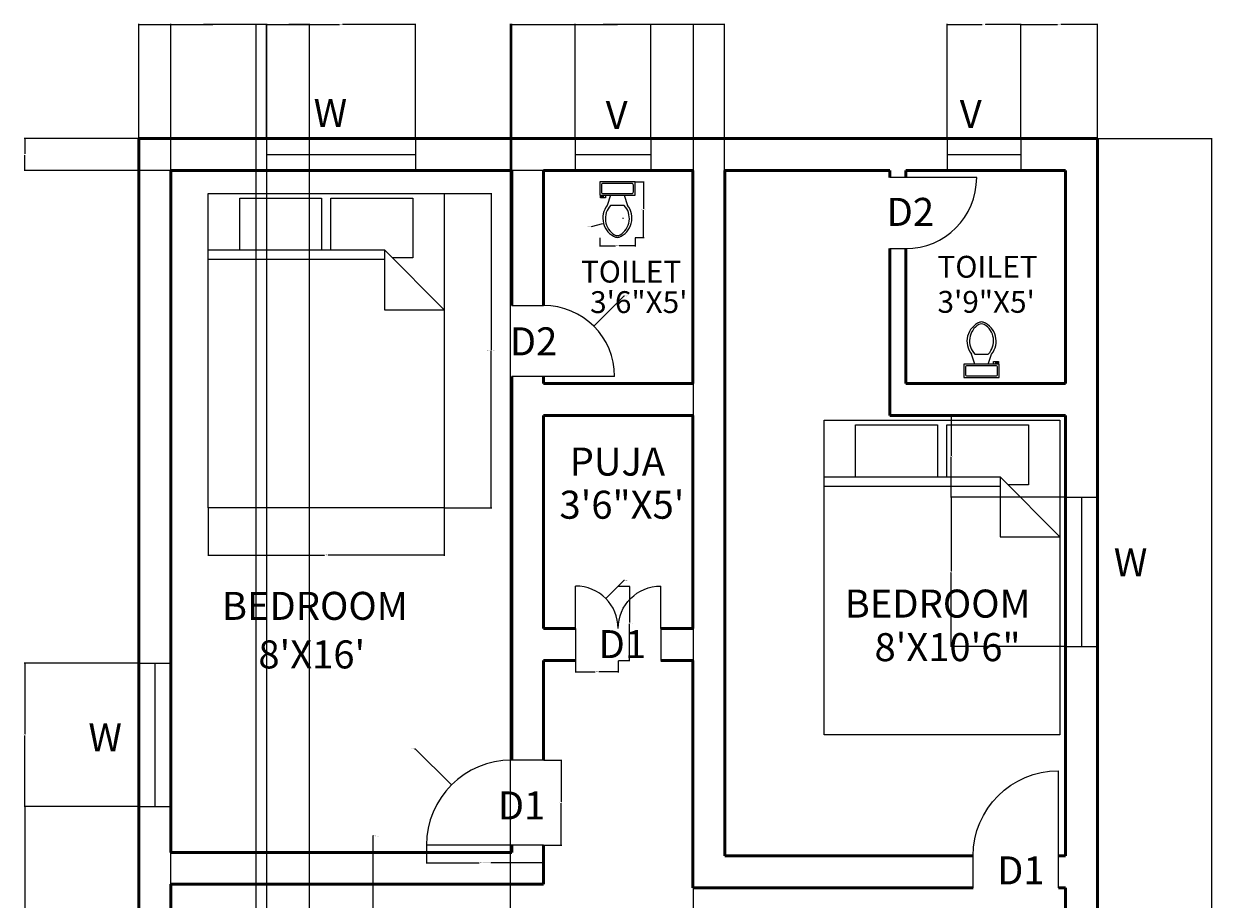
# Model space of a CAD drawing. Units: feet. Extents: x 1657 to 2001, y 1678 to 2367.
# Tile 4 of 4: x 1666 to 2001, y 2120 to 2367. Entities that reach past the tile are written whole.
import ezdxf

# ---------------------------------------------------------------- set-up
doc = ezdxf.new("R2010")
doc.units = ezdxf.units.FT
for name, color, linetype, lineweight in [('A-ANNO-DIMS', 2, 'Continuous', 18), ('A-ANNO-TEXT', 7, 'Continuous', 18), ('A-AREA-IDEN', 7, 'Continuous', 25), ('A-DOOR', 3, 'Continuous', 25), ('A-FLOR-FIXT', 8, 'Continuous', 18), ('A-FURN', 8, 'Continuous', 18), ('A-GLAZ', 4, 'Continuous', 18), ('A-WALL', 7, 'Continuous', 50)]:
    doc.layers.add(name, color=color, linetype=linetype, lineweight=lineweight)
doc.styles.get("Standard").update_dxf_attribs({"font": 'arial.ttf'})
doc.dimstyles.get("Standard").update_dxf_attribs({"dimtxt": 0.18, "dimasz": 0.18, "dimexe": 0.18, "dimexo": 0.0625, "dimgap": 0.09, "dimtad": 0, "dimtih": 1, "dimtoh": 1, "dimdec": 4, "dimzin": 0, "dimdsep": 46, "dimtxsty": 'Standard', "dimcen": 0.09, "dimadec": 0, "dimazin": 0, "dimtfac": 1, "dimtdec": 4, "dimtofl": 0, "dimtmove": 0, "dimatfit": 3, "dimfxl": 1, "dimtolj": 1, "dimtzin": 0, "dimarcsym": 0})

# ---------------------------------------------------------------- blocks, each defined once
blk = doc.blocks.new('Bed - Queen')
for p, q in [((0, -80.00003), (0, 0)), ((0, 0), (59.99999, 0)), ((59.99999, 0), (59.99999, -80.00003)), ((7.99999, -1.2), (28.79998, -1.2)), ((7.99999, -14.4), (7.99999, -1.2)), ((28.79998, -1.2), (28.79998, -14.4)), ((31.19999, -1.2), (51.99999, -1.2)), ((31.19999, -14.4), (31.19999, -1.2)), ((51.99999, -1.2), (51.99999, -16.4)), ((0, -14.4), (44.8, -14.4)), ((59.99999, -29.6), (44.8, -14.4)), ((44.8, -14.4), (44.8, -29.6)), ((44.8, -16.8), (0, -16.8)), ((51.99999, -16.4), (46.79936, -16.4)), ((44.8, -29.6), (59.99999, -29.6)), ((59.99999, -80.00003), (0, -80.00003))]:
    blk.add_line(p, q)
blk = doc.blocks.new('Toilet - top')
for p, q in [((9.5, -6), (9.5, -2)), ((-10, -8.5), (-8, -8.5)), ((-10, -9.5), (-10, -8.5)), ((-7, -9.5), (-10, -9.5)), ((-8, -8.5), (-8, -8)), ((-7, -8), (-7, -9.5)), ((-4, -8), (-6, -14)), ((4, -14), (-4, -14)), ((4, -8), (6, -14))]:
    blk.add_line(p, q)
blk.add_lwpolyline([(10.5, -8), (10.5, 0), (-10.5, 0), (-10.5, -8)], close=True)
for points in [[(-9.5, -2), (-9.5, -6)], [(8.5, -1), (-8.5, -1)], [(-8.5, -7), (8.5, -7)]]:
    blk.add_lwpolyline(points)
for centre, radius, start, end in [((-8.62, -1.88), 0.884, 81.8699, 188.1301), ((-8.62, -6.12), 0.884, 171.8699, 278.1301), ((8.62, -1.88), 0.884, 351.8699, 98.1301), ((8.62, -6.12), 0.884, 261.8699, 8.1301), ((3.52, -21.58), 12.17, 141.46911, 247.97143), ((4.2, -21.82), 11.33, 136.36773, 238.94682), ((-3.52, -21.58), 12.17, 292.02843, 38.53071), ((-4.2, -21.82), 11.33, 301.05301, 43.63209), ((0, -27.88), 4, 245.73182, 294.26817), ((0, -29), 4, 254.86053, 285.13947)]:
    blk.add_arc(centre, radius, start, end)
blk = doc.blocks.new('DOOR-BEDROOM-SINGLE')
for p, q in [((33, 24), (24, 24)), ((33, 0), (0, 0))]:
    blk.add_line(p, q)
blk.add_arc((24, 0), 24, 90, 180)
blk = doc.blocks.new('DOOR-PUJA-LEAF')
for q in [(0, 21), (0, 0)]:
    blk.add_line((0, 9), q)
blk.add_arc((0, 9), 12, 0, 90)
blk = doc.blocks.new('*D12')
at = {"layer": 'A-ANNO-DIMS', "color": 0, "lineweight": -2, "transparency": 16777216}
for p, q in [((1784.32, 2318.87), (1797.72, 2318.87)), ((1797.54, 2318.69), (1797.54, 2274.76)), ((1797.54, 2230.46), (1797.54, 2274.39)), ((1784.32, 2230.28), (1797.72, 2230.28))]:
    blk.add_line(p, q, dxfattribs=at)
at = {"layer": 'A-ANNO-DIMS', "color": 0, "transparency": 16777216}
for points in [[(1797.51, 2318.69), (1797.57, 2318.69), (1797.54, 2318.87)], [(1797.51, 2230.46), (1797.57, 2230.46), (1797.54, 2230.28)]]:
    blk.add_solid(points, dxfattribs=at)
at = {"layer": 'Defpoints', "color": 0, "transparency": 16777216}
for p in [(1784.26, 2318.87), (1797.54, 2318.87), (1784.26, 2230.28)]:
    blk.add_point(p, dxfattribs=at)
at = {"layer": 'A-ANNO-DIMS', "color": 0, "transparency": 16777216, "insert": (1797.54, 2274.57), "char_height": 0.18, "attachment_point": 5}
blk.add_mtext('\\A1;QUEEN BED 89 TYP.', dxfattribs=at)
blk = doc.blocks.new('*D13')
at = {"layer": 'A-ANNO-DIMS', "color": 0, "lineweight": -2, "transparency": 16777216}
for p, q in [((1717.81, 2230.22), (1717.81, 2216.81)), ((1784.26, 2230.22), (1784.26, 2216.81)), ((1717.99, 2216.99), (1750.51, 2216.99)), ((1784.08, 2216.99), (1751.56, 2216.99))]:
    blk.add_line(p, q, dxfattribs=at)
at = {"layer": 'A-ANNO-DIMS', "color": 0, "transparency": 16777216}
for points in [[(1717.99, 2217.02), (1717.99, 2216.96), (1717.81, 2216.99)], [(1784.08, 2217.02), (1784.08, 2216.96), (1784.26, 2216.99)]]:
    blk.add_solid(points, dxfattribs=at)
at = {"layer": 'Defpoints', "color": 0, "transparency": 16777216}
for p in [(1717.81, 2230.28), (1784.26, 2230.28), (1784.26, 2216.99)]:
    blk.add_point(p, dxfattribs=at)
at = {"layer": 'A-ANNO-DIMS', "color": 0, "transparency": 16777216, "insert": (1751.03, 2216.99), "char_height": 0.18, "attachment_point": 5}
blk.add_mtext('\\A1;66 TYP.', dxfattribs=at)
blk = doc.blocks.new('*D14')
at = {"layer": 'A-ANNO-DIMS', "color": 0, "lineweight": -2, "transparency": 16777216}
for p, q in [((1838.1, 2322.14), (1840.57, 2322.14)), ((1840.39, 2321.96), (1840.39, 2314.48)), ((1840.39, 2306.63), (1840.39, 2314.11)), ((1838.1, 2306.45), (1840.57, 2306.45))]:
    blk.add_line(p, q, dxfattribs=at)
at = {"layer": 'A-ANNO-DIMS', "color": 0, "transparency": 16777216}
for points in [[(1840.36, 2321.96), (1840.42, 2321.96), (1840.39, 2322.14)], [(1840.36, 2306.63), (1840.42, 2306.63), (1840.39, 2306.45)]]:
    blk.add_solid(points, dxfattribs=at)
at = {"layer": 'Defpoints', "color": 0, "transparency": 16777216}
for p in [(1838.04, 2322.14), (1840.39, 2322.14), (1838.04, 2306.45)]:
    blk.add_point(p, dxfattribs=at)
at = {"layer": 'A-ANNO-DIMS', "color": 0, "transparency": 16777216, "insert": (1840.39, 2314.3), "char_height": 0.18, "attachment_point": 5}
blk.add_mtext('\\A1;WC 16 TYP.', dxfattribs=at)
blk = doc.blocks.new('*D15')
at = {"layer": 'A-ANNO-DIMS', "color": 0, "lineweight": -2, "transparency": 16777216}
for p, q in [((1828.07, 2306.39), (1828.07, 2303.92)), ((1828.25, 2304.1), (1832.54, 2304.1)), ((1837.86, 2304.1), (1833.58, 2304.1)), ((1838.04, 2306.39), (1838.04, 2303.92))]:
    blk.add_line(p, q, dxfattribs=at)
at = {"layer": 'A-ANNO-DIMS', "color": 0, "transparency": 16777216}
for points in [[(1828.25, 2304.13), (1828.25, 2304.07), (1828.07, 2304.1)], [(1837.86, 2304.13), (1837.86, 2304.07), (1838.04, 2304.1)]]:
    blk.add_solid(points, dxfattribs=at)
at = {"layer": 'Defpoints', "color": 0, "transparency": 16777216}
for p in [(1828.07, 2306.45), (1838.04, 2306.45), (1838.04, 2304.1)]:
    blk.add_point(p, dxfattribs=at)
at = {"layer": 'A-ANNO-DIMS', "color": 0, "transparency": 16777216, "insert": (1833.06, 2304.1), "char_height": 0.18, "attachment_point": 5}
blk.add_mtext('\\A1;10 TYP.', dxfattribs=at)
blk = doc.blocks.new('*D28')
at = {"layer": 'A-ANNO-DIMS', "color": 0, "lineweight": -2, "transparency": 16777216}
for p, q in [((1779.28, 2135.24), (1779.28, 2130.17)), ((1812.28, 2135.24), (1812.28, 2130.17)), ((1779.46, 2130.35), (1794.16, 2130.35)), ((1812.1, 2130.35), (1797.41, 2130.35))]:
    blk.add_line(p, q, dxfattribs=at)
at = {"layer": 'A-ANNO-DIMS', "color": 0, "transparency": 16777216}
for points in [[(1779.46, 2130.38), (1779.46, 2130.32), (1779.28, 2130.35)], [(1812.1, 2130.38), (1812.1, 2130.32), (1812.28, 2130.35)]]:
    blk.add_solid(points, dxfattribs=at)
at = {"layer": 'Defpoints', "color": 0, "transparency": 16777216}
for p in [(1779.28, 2135.3), (1812.28, 2135.3), (1812.28, 2130.35)]:
    blk.add_point(p, dxfattribs=at)
at = {"layer": 'A-ANNO-DIMS', "color": 0, "transparency": 16777216, "insert": (1795.78, 2130.35), "char_height": 0.18, "attachment_point": 5}
blk.add_mtext('\\A1;BEDROOM DOOR 33 TYP.', dxfattribs=at)
blk = doc.blocks.new('*D29')
at = {"layer": 'A-ANNO-DIMS', "color": 0, "lineweight": -2, "transparency": 16777216}
for p, q in [((1812.35, 2159.3), (1817.41, 2159.3)), ((1817.23, 2159.12), (1817.23, 2147.48)), ((1817.23, 2135.48), (1817.23, 2147.12)), ((1812.35, 2135.3), (1817.41, 2135.3))]:
    blk.add_line(p, q, dxfattribs=at)
at = {"layer": 'A-ANNO-DIMS', "color": 0, "transparency": 16777216}
for points in [[(1817.2, 2159.12), (1817.26, 2159.12), (1817.23, 2159.3)], [(1817.2, 2135.48), (1817.26, 2135.48), (1817.23, 2135.3)]]:
    blk.add_solid(points, dxfattribs=at)
at = {"layer": 'Defpoints', "color": 0, "transparency": 16777216}
for p in [(1812.28, 2159.3), (1817.23, 2159.3), (1812.28, 2135.3)]:
    blk.add_point(p, dxfattribs=at)
at = {"layer": 'A-ANNO-DIMS', "color": 0, "transparency": 16777216, "insert": (1817.23, 2147.3), "char_height": 0.18, "attachment_point": 5}
blk.add_mtext('\\A1;24 TYP.', dxfattribs=at)
blk = doc.blocks.new('*D32')
at = {"layer": 'A-ANNO-DIMS', "color": 0, "lineweight": -2, "transparency": 16777216}
for p, q in [((1833.35, 2208.3), (1836.61, 2208.3)), ((1836.43, 2208.12), (1836.43, 2197.98)), ((1836.43, 2187.48), (1836.43, 2197.62)), ((1833.35, 2187.3), (1836.61, 2187.3))]:
    blk.add_line(p, q, dxfattribs=at)
at = {"layer": 'A-ANNO-DIMS', "color": 0, "transparency": 16777216}
for points in [[(1836.4, 2208.12), (1836.46, 2208.12), (1836.43, 2208.3)], [(1836.4, 2187.48), (1836.46, 2187.48), (1836.43, 2187.3)]]:
    blk.add_solid(points, dxfattribs=at)
at = {"layer": 'Defpoints', "color": 0, "transparency": 16777216}
for p in [(1833.28, 2208.3), (1836.43, 2208.3), (1833.28, 2187.3)]:
    blk.add_point(p, dxfattribs=at)
at = {"layer": 'A-ANNO-DIMS', "color": 0, "transparency": 16777216, "insert": (1836.43, 2197.8), "char_height": 0.18, "attachment_point": 5}
blk.add_mtext('\\A1;PUJA LEAF 21 TYP.', dxfattribs=at)
blk = doc.blocks.new('*D33')
at = {"layer": 'A-ANNO-DIMS', "color": 0, "lineweight": -2, "transparency": 16777216}
for p, q in [((1821.28, 2187.24), (1821.28, 2183.97)), ((1833.28, 2187.24), (1833.28, 2183.97)), ((1821.46, 2184.15), (1826.77, 2184.15)), ((1833.1, 2184.15), (1827.8, 2184.15))]:
    blk.add_line(p, q, dxfattribs=at)
at = {"layer": 'A-ANNO-DIMS', "color": 0, "transparency": 16777216}
for points in [[(1821.46, 2184.18), (1821.46, 2184.12), (1821.28, 2184.15)], [(1833.1, 2184.18), (1833.1, 2184.12), (1833.28, 2184.15)]]:
    blk.add_solid(points, dxfattribs=at)
at = {"layer": 'Defpoints', "color": 0, "transparency": 16777216}
for p in [(1821.28, 2187.3), (1833.28, 2187.3), (1833.28, 2184.15)]:
    blk.add_point(p, dxfattribs=at)
at = {"layer": 'A-ANNO-DIMS', "color": 0, "transparency": 16777216, "insert": (1827.28, 2184.15), "char_height": 0.18, "attachment_point": 5}
blk.add_mtext('\\A1;12 TYP.', dxfattribs=at)
blk = doc.blocks.new('*D35')
at = {"layer": 'A-ANNO-DIMS', "color": 0, "lineweight": -2, "transparency": 16777216}
for p, q in [((1968.35, 2334.3), (2000.61, 2334.3)), ((2000.43, 2334.12), (2000.43, 2022.48)), ((2000.43, 1710.48), (2000.43, 2022.12)), ((1968.35, 1710.3), (2000.61, 1710.3))]:
    blk.add_line(p, q, dxfattribs=at)
at = {"layer": 'A-ANNO-DIMS', "color": 0, "transparency": 16777216}
for points in [[(2000.4, 2334.12), (2000.46, 2334.12), (2000.43, 2334.3)], [(2000.4, 1710.48), (2000.46, 1710.48), (2000.43, 1710.3)]]:
    blk.add_solid(points, dxfattribs=at)
at = {"layer": 'Defpoints', "color": 0, "transparency": 16777216}
for p in [(1968.28, 2334.3), (2000.43, 2334.3), (1968.28, 1710.3)]:
    blk.add_point(p, dxfattribs=at)
at = {"layer": 'A-ANNO-DIMS', "color": 0, "transparency": 16777216, "insert": (2000.43, 2022.3), "char_height": 0.18, "attachment_point": 5}
blk.add_mtext('\\A1;624', dxfattribs=at)
blk = doc.blocks.new('*D37')
at = {"layer": 'A-ANNO-DIMS', "color": 0, "lineweight": -2, "transparency": 16777216}
for p, q in [((1734.28, 1770.36), (1734.28, 2366.63)), ((1734.46, 2366.45), (1740.08, 2366.45)), ((1746.1, 2366.45), (1740.49, 2366.45)), ((1746.28, 1770.36), (1746.28, 2366.63))]:
    blk.add_line(p, q, dxfattribs=at)
at = {"layer": 'A-ANNO-DIMS', "color": 0, "transparency": 16777216}
for points in [[(1734.46, 2366.48), (1734.46, 2366.42), (1734.28, 2366.45)], [(1746.1, 2366.48), (1746.1, 2366.42), (1746.28, 2366.45)]]:
    blk.add_solid(points, dxfattribs=at)
at = {"layer": 'Defpoints', "color": 0, "transparency": 16777216}
for p in [(1746.28, 2366.45), (1734.28, 1770.3), (1746.28, 1770.3)]:
    blk.add_point(p, dxfattribs=at)
at = {"layer": 'A-ANNO-DIMS', "color": 0, "transparency": 16777216, "insert": (1740.28, 2366.45), "char_height": 0.18, "attachment_point": 5}
blk.add_mtext('\\A1;12', dxfattribs=at)
blk = doc.blocks.new('*D38')
at = {"layer": 'A-ANNO-DIMS', "color": 0, "lineweight": -2, "transparency": 16777216}
for p, q in [((1698.28, 1770.36), (1698.28, 2366.63)), ((1698.46, 2366.45), (1716.07, 2366.45)), ((1734.1, 2366.45), (1716.5, 2366.45)), ((1734.28, 1770.36), (1734.28, 2366.63))]:
    blk.add_line(p, q, dxfattribs=at)
at = {"layer": 'A-ANNO-DIMS', "color": 0, "transparency": 16777216}
for points in [[(1698.46, 2366.48), (1698.46, 2366.42), (1698.28, 2366.45)], [(1734.1, 2366.48), (1734.1, 2366.42), (1734.28, 2366.45)]]:
    blk.add_solid(points, dxfattribs=at)
at = {"layer": 'Defpoints', "color": 0, "transparency": 16777216}
for p in [(1734.28, 2366.45), (1698.28, 1770.3), (1734.28, 1770.3)]:
    blk.add_point(p, dxfattribs=at)
at = {"layer": 'A-ANNO-DIMS', "color": 0, "transparency": 16777216, "insert": (1716.28, 2366.45), "char_height": 0.18, "attachment_point": 5}
blk.add_mtext('\\A1;36', dxfattribs=at)
blk = doc.blocks.new('*D39')
at = {"layer": 'A-ANNO-DIMS', "color": 0, "lineweight": -2, "transparency": 16777216}
for p, q in [((1698.28, 2334.36), (1698.28, 2366.63)), ((1698.46, 2366.45), (1715.79, 2366.45)), ((1734.04, 2366.45), (1716.72, 2366.45)), ((1734.22, 2334.36), (1734.22, 2366.63))]:
    blk.add_line(p, q, dxfattribs=at)
at = {"layer": 'A-ANNO-DIMS', "color": 0, "transparency": 16777216}
for points in [[(1698.46, 2366.48), (1698.46, 2366.42), (1698.28, 2366.45)], [(1734.04, 2366.48), (1734.04, 2366.42), (1734.22, 2366.45)]]:
    blk.add_solid(points, dxfattribs=at)
at = {"layer": 'Defpoints', "color": 0, "transparency": 16777216}
for p in [(1734.22, 2366.45), (1698.28, 2334.3), (1734.22, 2334.3)]:
    blk.add_point(p, dxfattribs=at)
at = {"layer": 'A-ANNO-DIMS', "color": 0, "transparency": 16777216, "insert": (1716.25, 2366.45), "char_height": 0.18, "attachment_point": 5}
blk.add_mtext('\\A1;35.935', dxfattribs=at)
blk = doc.blocks.new('*D40')
at = {"layer": 'A-ANNO-DIMS', "color": 0, "lineweight": -2, "transparency": 16777216}
for p, q in [((1734.22, 2334.36), (1734.22, 2366.63)), ((1734.4, 2366.45), (1754.79, 2366.45)), ((1775.98, 2366.45), (1755.59, 2366.45)), ((1776.16, 2334.36), (1776.16, 2366.63))]:
    blk.add_line(p, q, dxfattribs=at)
at = {"layer": 'A-ANNO-DIMS', "color": 0, "transparency": 16777216}
for points in [[(1734.4, 2366.48), (1734.4, 2366.42), (1734.22, 2366.45)], [(1775.98, 2366.48), (1775.98, 2366.42), (1776.16, 2366.45)]]:
    blk.add_solid(points, dxfattribs=at)
at = {"layer": 'Defpoints', "color": 0, "transparency": 16777216}
for p in [(1776.16, 2366.45), (1734.22, 2334.3), (1776.16, 2334.3)]:
    blk.add_point(p, dxfattribs=at)
at = {"layer": 'A-ANNO-DIMS', "color": 0, "transparency": 16777216, "insert": (1755.19, 2366.45), "char_height": 0.18, "attachment_point": 5}
blk.add_mtext('\\A1;41.94', dxfattribs=at)
blk = doc.blocks.new('*D41')
at = {"layer": 'A-ANNO-DIMS', "color": 0, "lineweight": -2, "transparency": 16777216}
for p, q in [((1925.97, 2334.36), (1925.97, 2366.63)), ((1926.15, 2366.45), (1935.87, 2366.45)), ((1946.52, 2366.45), (1936.8, 2366.45)), ((1946.7, 2334.36), (1946.7, 2366.63))]:
    blk.add_line(p, q, dxfattribs=at)
at = {"layer": 'A-ANNO-DIMS', "color": 0, "transparency": 16777216}
for points in [[(1926.15, 2366.48), (1926.15, 2366.42), (1925.97, 2366.45)], [(1946.52, 2366.48), (1946.52, 2366.42), (1946.7, 2366.45)]]:
    blk.add_solid(points, dxfattribs=at)
at = {"layer": 'Defpoints', "color": 0, "transparency": 16777216}
for p in [(1946.7, 2366.45), (1925.97, 2334.3), (1946.7, 2334.3)]:
    blk.add_point(p, dxfattribs=at)
at = {"layer": 'A-ANNO-DIMS', "color": 0, "transparency": 16777216, "insert": (1936.33, 2366.45), "char_height": 0.18, "attachment_point": 5}
blk.add_mtext('\\A1;20.726', dxfattribs=at)
blk = doc.blocks.new('*D42')
at = {"layer": 'A-ANNO-DIMS', "color": 0, "lineweight": -2, "transparency": 16777216}
for p, q in [((1946.7, 2334.36), (1946.7, 2366.63)), ((1946.88, 2366.45), (1957.03, 2366.45)), ((1968.1, 2366.45), (1957.96, 2366.45)), ((1968.28, 2334.36), (1968.28, 2366.63))]:
    blk.add_line(p, q, dxfattribs=at)
at = {"layer": 'A-ANNO-DIMS', "color": 0, "transparency": 16777216}
for points in [[(1946.88, 2366.48), (1946.88, 2366.42), (1946.7, 2366.45)], [(1968.1, 2366.48), (1968.1, 2366.42), (1968.28, 2366.45)]]:
    blk.add_solid(points, dxfattribs=at)
at = {"layer": 'Defpoints', "color": 0, "transparency": 16777216}
for p in [(1968.28, 2366.45), (1946.7, 2334.3), (1968.28, 2334.3)]:
    blk.add_point(p, dxfattribs=at)
at = {"layer": 'A-ANNO-DIMS', "color": 0, "transparency": 16777216, "insert": (1957.49, 2366.45), "char_height": 0.18, "attachment_point": 5}
blk.add_mtext('\\A1;21.588', dxfattribs=at)
blk = doc.blocks.new('*D46')
at = {"layer": 'A-ANNO-DIMS', "color": 0, "lineweight": -2, "transparency": 16777216}
for p, q in [((1698.22, 2146.17), (1665.95, 2146.17)), ((1666.13, 2145.99), (1666.13, 2111.13)), ((1666.13, 2075.91), (1666.13, 2110.77)), ((1698.22, 2075.73), (1665.95, 2075.73))]:
    blk.add_line(p, q, dxfattribs=at)
at = {"layer": 'A-ANNO-DIMS', "color": 0, "transparency": 16777216}
for points in [[(1666.1, 2145.99), (1666.16, 2145.99), (1666.13, 2146.17)], [(1666.1, 2075.91), (1666.16, 2075.91), (1666.13, 2075.73)]]:
    blk.add_solid(points, dxfattribs=at)
at = {"layer": 'Defpoints', "color": 0, "transparency": 16777216}
for p in [(1666.13, 2146.17), (1698.28, 2146.17), (1698.28, 2075.73)]:
    blk.add_point(p, dxfattribs=at)
at = {"layer": 'A-ANNO-DIMS', "color": 0, "transparency": 16777216, "insert": (1666.13, 2110.95), "char_height": 0.18, "attachment_point": 5}
blk.add_mtext('\\A1;70.44', dxfattribs=at)
blk = doc.blocks.new('*D47')
at = {"layer": 'A-ANNO-DIMS', "color": 0, "lineweight": -2, "transparency": 16777216}
for p, q in [((1698.22, 2186.61), (1665.95, 2186.61)), ((1666.13, 2186.43), (1666.13, 2166.57)), ((1666.13, 2146.35), (1666.13, 2166.21)), ((1698.22, 2146.17), (1665.95, 2146.17))]:
    blk.add_line(p, q, dxfattribs=at)
at = {"layer": 'A-ANNO-DIMS', "color": 0, "transparency": 16777216}
for points in [[(1666.1, 2186.43), (1666.16, 2186.43), (1666.13, 2186.61)], [(1666.1, 2146.35), (1666.16, 2146.35), (1666.13, 2146.17)]]:
    blk.add_solid(points, dxfattribs=at)
at = {"layer": 'Defpoints', "color": 0, "transparency": 16777216}
for p in [(1666.13, 2186.61), (1698.28, 2186.61), (1698.28, 2146.17)]:
    blk.add_point(p, dxfattribs=at)
at = {"layer": 'A-ANNO-DIMS', "color": 0, "transparency": 16777216, "insert": (1666.13, 2166.39), "char_height": 0.18, "attachment_point": 5}
blk.add_mtext('\\A1;40.45', dxfattribs=at)
blk = doc.blocks.new('*D48')
at = {"layer": 'A-ANNO-DIMS', "color": 0, "lineweight": -2, "transparency": 16777216}
for p, q in [((1959.22, 2233.29), (1926.95, 2233.29)), ((1927.13, 2233.11), (1927.13, 2212.44)), ((1927.13, 2191.4), (1927.13, 2212.07)), ((1959.22, 2191.22), (1926.95, 2191.22))]:
    blk.add_line(p, q, dxfattribs=at)
at = {"layer": 'A-ANNO-DIMS', "color": 0, "transparency": 16777216}
for points in [[(1927.1, 2233.11), (1927.16, 2233.11), (1927.13, 2233.29)], [(1927.1, 2191.4), (1927.16, 2191.4), (1927.13, 2191.22)]]:
    blk.add_solid(points, dxfattribs=at)
at = {"layer": 'Defpoints', "color": 0, "transparency": 16777216}
for p in [(1927.13, 2233.29), (1959.28, 2233.29), (1959.28, 2191.22)]:
    blk.add_point(p, dxfattribs=at)
at = {"layer": 'A-ANNO-DIMS', "color": 0, "transparency": 16777216, "insert": (1927.13, 2212.26), "char_height": 0.18, "attachment_point": 5}
blk.add_mtext('\\A1;42.06', dxfattribs=at)
blk = doc.blocks.new('*D49')
at = {"layer": 'A-ANNO-DIMS', "color": 0, "lineweight": -2, "transparency": 16777216}
for p, q in [((1959.22, 2256.3), (1926.95, 2256.3)), ((1927.13, 2256.12), (1927.13, 2244.97)), ((1927.13, 2233.47), (1927.13, 2244.61)), ((1959.22, 2233.29), (1926.95, 2233.29))]:
    blk.add_line(p, q, dxfattribs=at)
at = {"layer": 'A-ANNO-DIMS', "color": 0, "transparency": 16777216}
for points in [[(1927.1, 2256.12), (1927.16, 2256.12), (1927.13, 2256.3)], [(1927.1, 2233.47), (1927.16, 2233.47), (1927.13, 2233.29)]]:
    blk.add_solid(points, dxfattribs=at)
at = {"layer": 'Defpoints', "color": 0, "transparency": 16777216}
for p in [(1927.13, 2256.3), (1959.28, 2256.3), (1959.28, 2233.29)]:
    blk.add_point(p, dxfattribs=at)
at = {"layer": 'A-ANNO-DIMS', "color": 0, "transparency": 16777216, "insert": (1927.13, 2244.79), "char_height": 0.18, "attachment_point": 5}
blk.add_mtext('\\A1;23.01', dxfattribs=at)
blk = doc.blocks.new('*D50')
at = {"layer": 'A-ANNO-DIMS', "color": 0, "lineweight": -2, "transparency": 16777216}
for p, q in [((1803.28, 2325.36), (1803.28, 2366.63)), ((1803.46, 2366.45), (1833.07, 2366.45)), ((1863.1, 2366.45), (1833.5, 2366.45)), ((1863.28, 2325.36), (1863.28, 2366.63))]:
    blk.add_line(p, q, dxfattribs=at)
at = {"layer": 'A-ANNO-DIMS', "color": 0, "transparency": 16777216}
for points in [[(1803.46, 2366.48), (1803.46, 2366.42), (1803.28, 2366.45)], [(1863.1, 2366.48), (1863.1, 2366.42), (1863.28, 2366.45)]]:
    blk.add_solid(points, dxfattribs=at)
at = {"layer": 'Defpoints', "color": 0, "transparency": 16777216}
for p in [(1863.28, 2366.45), (1803.28, 2325.3), (1863.28, 2325.3)]:
    blk.add_point(p, dxfattribs=at)
at = {"layer": 'A-ANNO-DIMS', "color": 0, "transparency": 16777216, "insert": (1833.28, 2366.45), "char_height": 0.18, "attachment_point": 5}
blk.add_mtext('\\A1;60', dxfattribs=at)
blk = doc.blocks.new('*D51')
at = {"layer": 'A-ANNO-DIMS', "color": 0, "lineweight": -2, "transparency": 16777216}
for p, q in [((1821.17, 2334.36), (1821.17, 2366.63)), ((1821.35, 2366.45), (1831.45, 2366.45)), ((1842.34, 2366.45), (1832.24, 2366.45)), ((1842.52, 2334.36), (1842.52, 2366.63))]:
    blk.add_line(p, q, dxfattribs=at)
at = {"layer": 'A-ANNO-DIMS', "color": 0, "transparency": 16777216}
for points in [[(1821.35, 2366.48), (1821.35, 2366.42), (1821.17, 2366.45)], [(1842.34, 2366.48), (1842.34, 2366.42), (1842.52, 2366.45)]]:
    blk.add_solid(points, dxfattribs=at)
at = {"layer": 'Defpoints', "color": 0, "transparency": 16777216}
for p in [(1842.52, 2366.45), (1821.17, 2334.3), (1842.52, 2334.3)]:
    blk.add_point(p, dxfattribs=at)
at = {"layer": 'A-ANNO-DIMS', "color": 0, "transparency": 16777216, "insert": (1831.85, 2366.45), "char_height": 0.18, "attachment_point": 5}
blk.add_mtext('\\A1;21.35', dxfattribs=at)
blk = doc.blocks.new('*D52')
at = {"layer": 'A-ANNO-DIMS', "color": 0, "lineweight": -2, "transparency": 16777216}
for p, q in [((1821.11, 2334.3), (1665.95, 2334.3)), ((1666.13, 2334.12), (1666.13, 2329.98)), ((1666.13, 2325.48), (1666.13, 2329.62)), ((1821.11, 2325.3), (1665.95, 2325.3))]:
    blk.add_line(p, q, dxfattribs=at)
at = {"layer": 'A-ANNO-DIMS', "color": 0, "transparency": 16777216}
for points in [[(1666.1, 2334.12), (1666.16, 2334.12), (1666.13, 2334.3)], [(1666.1, 2325.48), (1666.16, 2325.48), (1666.13, 2325.3)]]:
    blk.add_solid(points, dxfattribs=at)
at = {"layer": 'Defpoints', "color": 0, "transparency": 16777216}
for p in [(1821.17, 2334.3), (1666.13, 2325.3), (1821.17, 2325.3)]:
    blk.add_point(p, dxfattribs=at)
at = {"layer": 'A-ANNO-DIMS', "color": 0, "transparency": 16777216, "insert": (1666.13, 2329.8), "char_height": 0.18, "attachment_point": 5}
blk.add_mtext('\\A1;9', dxfattribs=at)
blk = doc.blocks.new('*D55')
at = {"layer": 'A-ANNO-DIMS', "color": 0, "lineweight": -2, "transparency": 16777216}
for p, q in [((1707.28, 1851.36), (1707.28, 2366.63)), ((1707.46, 2366.45), (1719.06, 2366.45)), ((1731.1, 2366.45), (1719.5, 2366.45)), ((1731.28, 1851.36), (1731.28, 2366.63))]:
    blk.add_line(p, q, dxfattribs=at)
at = {"layer": 'A-ANNO-DIMS', "color": 0, "transparency": 16777216}
for points in [[(1707.46, 2366.48), (1707.46, 2366.42), (1707.28, 2366.45)], [(1731.1, 2366.48), (1731.1, 2366.42), (1731.28, 2366.45)]]:
    blk.add_solid(points, dxfattribs=at)
at = {"layer": 'Defpoints', "color": 0, "transparency": 16777216}
for p in [(1731.28, 2366.45), (1707.28, 1851.3), (1731.28, 1851.3)]:
    blk.add_point(p, dxfattribs=at)
at = {"layer": 'A-ANNO-DIMS', "color": 0, "transparency": 16777216, "insert": (1719.28, 2366.45), "char_height": 0.18, "attachment_point": 5}
blk.add_mtext('\\A1;24', dxfattribs=at)
blk = doc.blocks.new('*D56')
at = {"layer": 'A-ANNO-DIMS', "color": 0, "lineweight": -2, "transparency": 16777216}
for p, q in [((1802.91, 1992.36), (1802.91, 2366.63)), ((1803.09, 2366.45), (1828.29, 2366.45)), ((1854.28, 2366.45), (1829.08, 2366.45)), ((1854.46, 1992.36), (1854.46, 2366.63))]:
    blk.add_line(p, q, dxfattribs=at)
at = {"layer": 'A-ANNO-DIMS', "color": 0, "transparency": 16777216}
for points in [[(1803.09, 2366.48), (1803.09, 2366.42), (1802.91, 2366.45)], [(1854.28, 2366.48), (1854.28, 2366.42), (1854.46, 2366.45)]]:
    blk.add_solid(points, dxfattribs=at)
at = {"layer": 'Defpoints', "color": 0, "transparency": 16777216}
for p in [(1854.46, 2366.45), (1802.91, 1992.3), (1854.46, 1992.3)]:
    blk.add_point(p, dxfattribs=at)
at = {"layer": 'A-ANNO-DIMS', "color": 0, "transparency": 16777216, "insert": (1828.68, 2366.45), "char_height": 0.18, "attachment_point": 5}
blk.add_mtext('\\A1;51.55', dxfattribs=at)
blk = doc.blocks.new('*D60')
at = {"layer": 'A-ANNO-DIMS', "color": 0, "lineweight": -2, "transparency": 16777216}
for p, q in [((1775.95, 2162.45), (1776.13, 2162.45)), ((1776.13, 2162.45), (1786.19, 2152.4)), ((1803.19, 2135.3), (1803.37, 2135.3)), ((1803.28, 2135.21), (1803.28, 2135.39))]:
    blk.add_line(p, q, dxfattribs=at)
at = {"layer": 'A-ANNO-DIMS', "color": 0, "transparency": 16777216}
blk.add_solid([(1786.21, 2152.42), (1786.17, 2152.37), (1786.31, 2152.27)], dxfattribs=at)
at = {"layer": 'Defpoints', "color": 0, "transparency": 16777216}
for p in [(1786.31, 2152.27), (1803.28, 2135.3)]:
    blk.add_point(p, dxfattribs=at)
at = {"layer": 'A-ANNO-DIMS', "color": 0, "transparency": 16777216, "insert": (1775.45, 2162.45), "char_height": 0.18, "attachment_point": 5}
blk.add_mtext('\\A1;2X R24', dxfattribs=at)
blk = doc.blocks.new('*D61')
at = {"layer": 'A-ANNO-DIMS', "color": 0, "lineweight": -2, "transparency": 16777216}
for p, q in [((1834.91, 2289.93), (1826.55, 2281.57)), ((1835.09, 2289.93), (1834.91, 2289.93)), ((1812.19, 2267.3), (1812.37, 2267.3)), ((1812.28, 2267.21), (1812.28, 2267.39))]:
    blk.add_line(p, q, dxfattribs=at)
at = {"layer": 'A-ANNO-DIMS', "color": 0, "transparency": 16777216}
blk.add_solid([(1826.53, 2281.59), (1826.58, 2281.55), (1826.43, 2281.44)], dxfattribs=at)
at = {"layer": 'Defpoints', "color": 0, "transparency": 16777216}
for p in [(1826.43, 2281.44), (1812.28, 2267.3)]:
    blk.add_point(p, dxfattribs=at)
at = {"layer": 'A-ANNO-DIMS', "color": 0, "transparency": 16777216, "insert": (1835.59, 2289.93), "char_height": 0.18, "attachment_point": 5}
blk.add_mtext('\\A1;2X R20', dxfattribs=at)
blk = doc.blocks.new('*D62')
at = {"layer": 'A-ANNO-DIMS', "color": 0, "lineweight": -2, "transparency": 16777216}
for p, q in [((1834.86, 2209.87), (1829.9, 2204.91)), ((1835.04, 2209.87), (1834.86, 2209.87)), ((1821.28, 2196.21), (1821.28, 2196.39)), ((1821.19, 2196.3), (1821.37, 2196.3))]:
    blk.add_line(p, q, dxfattribs=at)
at = {"layer": 'A-ANNO-DIMS', "color": 0, "transparency": 16777216}
blk.add_solid([(1829.88, 2204.93), (1829.92, 2204.89), (1829.77, 2204.78)], dxfattribs=at)
at = {"layer": 'Defpoints', "color": 0, "transparency": 16777216}
for p in [(1829.77, 2204.78), (1821.28, 2196.3)]:
    blk.add_point(p, dxfattribs=at)
at = {"layer": 'A-ANNO-DIMS', "color": 0, "transparency": 16777216, "insert": (1835.54, 2209.87), "char_height": 0.18, "attachment_point": 5}
blk.add_mtext('\\A1;2X R12', dxfattribs=at)
blk = doc.blocks.new('*D65')
at = {"layer": 'A-ANNO-DIMS', "color": 0, "lineweight": -2, "transparency": 16777216}
for p, q in [((1764.33, 2137.91), (1764.15, 2137.91)), ((1764.15, 2137.91), (1764.15, 2115.43)), ((1764.06, 2077.47), (1764.24, 2077.47)), ((1764.15, 2077.38), (1764.15, 2077.56))]:
    blk.add_line(p, q, dxfattribs=at)
at = {"layer": 'A-ANNO-DIMS', "color": 0, "transparency": 16777216}
blk.add_solid([(1764.12, 2115.43), (1764.18, 2115.43), (1764.15, 2115.25)], dxfattribs=at)
at = {"layer": 'Defpoints', "color": 0, "transparency": 16777216}
for p in [(1764.15, 2115.25), (1764.15, 2077.47)]:
    blk.add_point(p, dxfattribs=at)
at = {"layer": 'A-ANNO-DIMS', "color": 0, "transparency": 16777216, "insert": (1765.07, 2137.91), "char_height": 0.18, "attachment_point": 5}
blk.add_mtext('\\A1;2X R37.776', dxfattribs=at)
blk = doc.blocks.new('*D67')
at = {"layer": 'A-ANNO-DIMS', "color": 0, "lineweight": -2, "transparency": 16777216}
for p, q in [((1825.79, 2309.55), (1828.97, 2310.38)), ((1834.64, 2311.9), (1834.82, 2311.9)), ((1834.73, 2311.81), (1834.73, 2311.99))]:
    blk.add_line(p, q, dxfattribs=at)
at = {"layer": 'A-ANNO-DIMS', "color": 0, "transparency": 16777216}
blk.add_solid([(1828.96, 2310.41), (1828.98, 2310.35), (1829.14, 2310.43)], dxfattribs=at)
at = {"layer": 'Defpoints', "color": 0, "transparency": 16777216}
for p in [(1829.14, 2310.43), (1834.73, 2311.9)]:
    blk.add_point(p, dxfattribs=at)
at = {"layer": 'A-ANNO-DIMS', "color": 0, "transparency": 16777216, "insert": (1825.11, 2309.55), "char_height": 0.18, "attachment_point": 5}
blk.add_mtext('\\A1;4X R5.775', dxfattribs=at)

msp = doc.modelspace()

# ---------------------------------------------------------------- linework, layer by layer
at = {"layer": 'A-DOOR'}
for p, q in [((1934.2848, 2323.2977), (1909.7848, 2323.2977)), ((1909.7848, 2303.2977), (1914.2848, 2303.2977)), ((1803.2848, 2287.2977), (1812.2848, 2287.2977)), ((1832.2848, 2267.2977), (1803.2848, 2267.2977))]:
    msp.add_line(p, q, dxfattribs=at)
for centre, start, end in [((1914.2848, 2323.2977), 270, 360), ((1812.2848, 2267.2977), 0, 90)]:
    msp.add_arc(centre, 20, start, end, dxfattribs=at)
at = {"layer": 'A-GLAZ'}
for p, q in [((1734.2201, 2334.2977), (1734.2201, 2325.2977)), ((1776.1583, 2334.2977), (1776.1583, 2325.2977)), ((1821.172, 2334.2977), (1821.172, 2325.2977)), ((1842.5209, 2334.2977), (1842.5209, 2325.2977)), ((1925.971, 2334.2977), (1925.971, 2325.2977)), ((1946.6972, 2334.2977), (1946.6972, 2325.2977)), ((1734.2201, 2329.7977), (1776.1583, 2329.7977)), ((1821.172, 2329.7977), (1842.5209, 2329.7977)), ((1925.971, 2329.7977), (1946.6972, 2329.7977)), ((1959.2848, 2233.2864), (1968.2848, 2233.2864)), ((1963.7848, 2233.2864), (1963.7848, 2191.2246)), ((1959.2848, 2191.2246), (1968.2848, 2191.2246)), ((1698.2848, 2186.6116), (1707.2848, 2186.6116)), ((1702.7848, 2186.6116), (1702.7848, 2146.1652)), ((1698.2848, 2146.1652), (1707.2848, 2146.1652))]:
    msp.add_line(p, q, dxfattribs=at)
at = {"layer": 'A-WALL'}
for p, q in [((1698.2848, 2334.2977), (1968.2848, 2334.2977)), ((1698.2848, 2133.2977), (1698.2848, 2334.2977)), ((1698.2848, 2334.2977), (1698.2848, 1842.2977)), ((1812.2848, 2334.2977), (1854.2848, 2334.2977)), ((1968.2848, 2334.2977), (1914.2848, 2334.2977)), ((1968.2848, 2265.2977), (1968.2848, 2334.2977)), ((1968.2848, 2132.2751), (1968.2848, 2334.2977)), ((1968.2848, 2334.2977), (1968.2848, 1983.2977)), ((1707.2848, 2325.2977), (1803.2848, 2325.2977)), ((1707.2848, 2133.2977), (1707.2848, 2325.2977)), ((1803.2848, 2325.2977), (1803.2848, 2287.2977)), ((1812.2848, 2325.2977), (1812.2848, 2287.2977)), ((1812.2848, 2325.2977), (1854.2848, 2325.2977)), ((1854.2848, 2325.2977), (1854.2848, 2265.2977)), ((1863.2848, 2325.2977), (1863.2848, 2132.2751)), ((1863.2848, 2325.2977), (1909.7848, 2325.2977)), ((1909.7848, 2325.2977), (1909.7848, 2323.2977)), ((1959.2848, 2325.2977), (1914.2848, 2325.2977)), ((1914.2848, 2325.2977), (1914.2848, 2323.2977)), ((1959.2848, 2265.2977), (1959.2848, 2325.2977)), ((1909.7848, 2303.2977), (1909.7848, 2256.2977)), ((1914.2848, 2303.2977), (1914.2848, 2265.2977)), ((1803.2848, 2267.2977), (1803.2848, 2159.2977)), ((1812.2848, 2267.2977), (1812.2848, 2265.2977)), ((1854.2848, 2265.2977), (1812.2848, 2265.2977)), ((1914.2848, 2265.2977), (1959.2848, 2265.2977)), ((1854.2848, 2256.2977), (1812.2848, 2256.2977)), ((1812.2848, 2256.2977), (1812.2848, 2196.2977)), ((1854.2848, 2256.2977), (1854.2848, 2196.2977)), ((1863.2848, 2256.2977), (1863.2848, 2196.2977)), ((1959.2848, 2256.2977), (1909.7848, 2256.2977)), ((1959.2848, 2132.2751), (1959.2848, 2256.2977)), ((1821.2848, 2196.2977), (1812.2848, 2196.2977)), ((1854.2848, 2196.2977), (1845.2848, 2196.2977)), ((1863.2848, 2196.2977), (1863.2848, 2132.2751)), ((1812.2848, 2187.2977), (1812.2848, 2159.2977)), ((1821.2848, 2187.2977), (1812.2848, 2187.2977)), ((1854.2848, 2187.2977), (1845.2848, 2187.2977)), ((1854.2848, 2187.2977), (1854.2848, 2123.2751)), ((1803.2848, 2133.2977), (1707.2848, 2133.2977)), ((1803.2848, 2135.2977), (1803.2848, 2133.2977)), ((1812.2848, 2135.2977), (1812.2848, 2124.2977)), ((1863.2848, 2132.2751), (1933.2848, 2132.2751)), ((1957.2848, 2132.2751), (1959.2848, 2132.2751)), ((1812.2848, 2124.2977), (1707.2848, 2124.2977)), ((1707.2848, 2124.2977), (1707.2848, 1992.2977)), ((1854.2848, 2123.2751), (1933.2848, 2123.2751)), ((1957.2848, 2123.2751), (1959.2848, 2123.2751)), ((1959.2848, 2123.2751), (1959.2848, 1992.2977))]:
    msp.add_line(p, q, dxfattribs=at)

# ---------------------------------------------------------------- block references
at = {"layer": 'A-DOOR'}
for name, p in [('DOOR-PUJA-LEAF', (1821.285, 2187.298)), ('DOOR-BEDROOM-SINGLE', (1779.285, 2135.298))]:
    msp.add_blockref(name, p, dxfattribs=at)
at = {"layer": 'A-DOOR', "extrusion": (0, 0, -1), "zscale": -1}
msp.add_blockref('DOOR-PUJA-LEAF', (-1845.2845, 2187.298), dxfattribs=at)
at = {"layer": 'A-DOOR', "extrusion": (0, 0, -1), "zscale": -1, "rotation": 270.0000000000002}
msp.add_blockref('DOOR-BEDROOM-SINGLE', (-1957.2844, 2156.2749), dxfattribs=at)
at = {"layer": 'A-FLOR-FIXT', "xscale": 0.4745993558592044, "yscale": 0.4745993558592044, "zscale": 0.4745993558592044}
msp.add_blockref('Toilet - top', (1833.0572, 2322.1378), dxfattribs=at)
at = {"layer": 'A-FLOR-FIXT', "xscale": 0.4745993558592044, "yscale": 0.4745993558592044, "zscale": 0.4745993558592044, "rotation": 180}
msp.add_blockref('Toilet - top', (1935.6529, 2266.9871), dxfattribs=at)
at = {"layer": 'A-FURN', "xscale": 1.107372928560116, "yscale": 1.107372928560116, "zscale": 1.107372928560116}
for p in [(1717.8129, 2318.8686), (1891.3071, 2254.9704)]:
    msp.add_blockref('Bed - Queen', p, dxfattribs=at)

# ---------------------------------------------------------------- texts
at = {"layer": 'A-ANNO-TEXT'}
for s, height, p in [('W', 7.8904, (1747.4844, 2337.5871)), ('V', 7.8904, (1829.7555, 2337.0236)), ('V', 7.8904, (1929.5065, 2337.2886)), ('D2', 7.89038, (1908.907, 2309.7051)), ('D2', 7.89038, (1802.7542, 2273.2496)), ('W', 7.8904, (1972.9158, 2210.9843)), ('D1', 7.89038, (1827.7642, 2187.9876)), ('W', 7.8904, (1684.0358, 2161.735)), ('D1', 7.89038, (1799.3738, 2142.5588)), ('D1', 7.89038, (1940.0407, 2124.2734))]:
    msp.add_text(s, height=height, dxfattribs=at).set_placement(p)
at = {"layer": 'A-AREA-IDEN'}
for s, height, p in [('TOILET', 6.15244, (1923.2424, 2295.1248)), ('TOILET', 6.15244, (1822.7875, 2293.7515)), ('3\'6"X5\'', 6.15244, (1825.3767, 2285.1717)), ('3\'9"X5\'', 6.15244, (1923.2424, 2285.2415)), ('PUJA', 7.89038, (1819.6235, 2239.3965)), ('3\'6"X5\'', 7.89038, (1816.7506, 2227.2432)), ('BEDROOM', 7.89038, (1721.6395, 2198.7619)), ('BEDROOM', 7.89038, (1897.0977, 2199.3998)), ("8'X16'", 7.89038, (1731.9256, 2185.0921)), ('8\'X10\'6"', 7.89038, (1905.4994, 2187.1375))]:
    msp.add_text(s, height=height, dxfattribs=at).set_placement(p)

# ---------------------------------------------------------------- dimensions: what is measured, and where the dimension line sits
at = {"layer": 'A-ANNO-DIMS'}
for base, p1, p2, override, picture, middle in [((1734.2848, 2366.4477), (1698.2848, 1770.2977), (1734.2848, 1770.2977), {"dimdec": 0, "dimlfac": 1, "dimrnd": 0, "dimzin": 0, "dimdsep": 46, "dimlunit": 2}, '*D38', (1716.2848, 2366.4477)), ((1734.2201, 2366.4477), (1698.2848, 2334.2977), (1734.2201, 2334.2977), {"dimdec": 3, "dimlfac": 1, "dimrnd": 0, "dimzin": 0, "dimdsep": 46, "dimlunit": 2}, '*D39', (1716.2524, 2366.4477)), ((1731.2848, 2366.4477), (1707.2848, 1851.2977), (1731.2848, 1851.2977), {"dimdec": 0, "dimlfac": 1, "dimrnd": 0, "dimzin": 0, "dimdsep": 46, "dimlunit": 2}, '*D55', (1719.2848, 2366.4477)), ((1776.1583, 2366.4477), (1734.2201, 2334.2977), (1776.1583, 2334.2977), {"dimdec": 2, "dimlfac": 1, "dimrnd": 0, "dimzin": 0, "dimdsep": 46, "dimlunit": 2}, '*D40', (1755.1892, 2366.4477)), ((1746.2848, 2366.4477), (1734.2848, 1770.2977), (1746.2848, 1770.2977), {"dimdec": 0, "dimlfac": 1, "dimrnd": 0, "dimzin": 0, "dimdsep": 46, "dimlunit": 2}, '*D37', (1740.2848, 2366.4477)), ((1854.4579, 2366.4477), (1802.9077, 1992.2977), (1854.4579, 1992.2977), {"dimdec": 2, "dimlfac": 1, "dimrnd": 0, "dimzin": 0, "dimdsep": 46, "dimlunit": 2}, '*D56', (1828.6828, 2366.4477)), ((1863.2848, 2366.4477), (1803.2848, 2325.2977), (1863.2848, 2325.2977), {"dimdec": 0, "dimlfac": 1, "dimrnd": 0, "dimzin": 0, "dimdsep": 46, "dimlunit": 2}, '*D50', (1833.2848, 2366.4477)), ((1842.5209, 2366.4477), (1821.172, 2334.2977), (1842.5209, 2334.2977), {"dimdec": 2, "dimlfac": 1, "dimrnd": 0, "dimzin": 0, "dimdsep": 46, "dimlunit": 2}, '*D51', (1831.8465, 2366.4477)), ((1946.6972, 2366.4477), (1925.971, 2334.2977), (1946.6972, 2334.2977), {"dimdec": 3, "dimlfac": 1, "dimrnd": 0, "dimzin": 0, "dimdsep": 46, "dimlunit": 2}, '*D41', (1936.3341, 2366.4477)), ((1968.2848, 2366.4477), (1946.6972, 2334.2977), (1968.2848, 2334.2977), {"dimdec": 3, "dimlfac": 1, "dimrnd": 0, "dimzin": 0, "dimdsep": 46, "dimlunit": 2}, '*D42', (1957.491, 2366.4477))]:
    dim = msp.add_linear_dim(base=base, p1=p1, p2=p2, dimstyle='Standard', override=override, dxfattribs=at)
    dim.commit()
    dim.dimension.update_dxf_attribs({"geometry": picture, "text_midpoint": middle})
for base, p1, p2, override, picture, middle in [((1666.1348, 2325.2977), (1821.172, 2334.2977), (1821.172, 2325.2977), {"dimdec": 0, "dimlfac": 1, "dimrnd": 0, "dimzin": 0, "dimdsep": 46, "dimlunit": 2}, '*D52', (1666.1348, 2329.7977)), ((2000.4348, 2334.2977), (1968.2848, 1710.2977), (1968.2848, 2334.2977), {"dimdec": 0, "dimlfac": 1, "dimrnd": 0, "dimzin": 0, "dimdsep": 46, "dimlunit": 2}, '*D35', (2000.4348, 2022.2977)), ((1927.1348, 2256.2977), (1959.2848, 2233.2864), (1959.2848, 2256.2977), {"dimdec": 2, "dimlfac": 1, "dimrnd": 0, "dimzin": 0, "dimdsep": 46, "dimlunit": 2}, '*D49', (1927.1348, 2244.792)), ((1927.1348, 2233.2864), (1959.2848, 2191.2246), (1959.2848, 2233.2864), {"dimdec": 2, "dimlfac": 1, "dimrnd": 0, "dimzin": 0, "dimdsep": 46, "dimlunit": 2}, '*D48', (1927.1348, 2212.2555)), ((1666.1348, 2186.6116), (1698.2848, 2146.1652), (1698.2848, 2186.6116), {"dimdec": 2, "dimlfac": 1, "dimrnd": 0, "dimzin": 0, "dimdsep": 46, "dimlunit": 2}, '*D47', (1666.1348, 2166.3884)), ((1666.1348, 2146.1652), (1698.2848, 2075.729), (1698.2848, 2146.1652), {"dimdec": 2, "dimlfac": 1, "dimrnd": 0, "dimzin": 0, "dimdsep": 46, "dimlunit": 2}, '*D46', (1666.1348, 2110.9471))]:
    dim = msp.add_linear_dim(base=base, p1=p1, p2=p2, angle=90, dimstyle='Standard', override=override, dxfattribs=at)
    dim.commit()
    dim.dimension.update_dxf_attribs({"geometry": picture, "text_midpoint": middle})
for base, p1, p2, text, picture, middle in [((1840.393, 2322.1378), (1838.0405, 2306.4541), (1838.0405, 2322.1378), 'WC <> TYP.', '*D14', (1840.393, 2314.296)), ((1797.5437, 2318.8686), (1784.2552, 2230.2787), (1784.2552, 2318.8686), 'QUEEN BED <> TYP.', '*D12', (1797.5437, 2274.5737)), ((1836.4348, 2208.2977), (1833.2848, 2187.2977), (1833.2848, 2208.2977), 'PUJA LEAF <> TYP.', '*D32', (1836.4348, 2197.7977)), ((1817.2348, 2159.2977), (1812.2848, 2135.2977), (1812.2848, 2159.2977), '<> TYP.', '*D29', (1817.2348, 2147.2977))]:
    dim = msp.add_linear_dim(base=base, p1=p1, p2=p2, angle=90, text=text, dimstyle='Standard', override={"dimdec": 0, "dimlfac": 1, "dimrnd": 0, "dimzin": 0, "dimdsep": 46, "dimlunit": 2}, dxfattribs=at)
    dim.commit()
    dim.dimension.update_dxf_attribs({"geometry": picture, "text_midpoint": middle})
for center, mpoint, text, override, picture, middle in [((1834.7276, 2311.8958), (1829.1418, 2310.4279), '4X <>', {"dimdec": 3, "dimlfac": 1, "dimrnd": 0, "dimzin": 0, "dimdsep": 46, "dimlunit": 2}, '*D67', (1825.7903, 2309.5473)), ((1812.2848, 2267.2977), (1826.4268, 2281.4398), '2X <>', {"dimdec": 0, "dimlfac": 1, "dimrnd": 0, "dimzin": 0, "dimdsep": 46, "dimlunit": 2}, '*D61', (1835.5918, 2289.9252)), ((1821.2848, 2196.2977), (1829.77, 2204.783), '2X <>', {"dimdec": 0, "dimlfac": 1, "dimrnd": 0, "dimzin": 0, "dimdsep": 46, "dimlunit": 2}, '*D62', (1835.5402, 2209.8742)), ((1803.2848, 2135.2977), (1786.314, 2152.268), '2X <>', {"dimdec": 0, "dimlfac": 1, "dimrnd": 0, "dimzin": 0, "dimdsep": 46, "dimlunit": 2}, '*D60', (1775.4519, 2162.4502)), ((1764.1489, 2077.471), (1764.149, 2115.2469), '2X <>', {"dimdec": 3, "dimlfac": 1, "dimrnd": 0, "dimzin": 0, "dimdsep": 46, "dimlunit": 2}, '*D65', (1765.0737, 2137.9125))]:
    dim = msp.add_radius_dim(center=center, mpoint=mpoint, text=text, dimstyle='Standard', override=override, dxfattribs=at)
    dim.commit()
    dim.dimension.update_dxf_attribs({"geometry": picture, "text_midpoint": middle, "dimtype": 164})
for base, p1, p2, text, picture, middle in [((1838.0405, 2304.1016), (1828.0739, 2306.4541), (1838.0405, 2306.4541), '<> TYP.', '*D15', (1833.0572, 2304.1016)), ((1784.2552, 2216.9902), (1717.8129, 2230.2787), (1784.2552, 2230.2787), '<> TYP.', '*D13', (1751.034, 2216.9902)), ((1833.2848, 2184.1477), (1821.2848, 2187.2977), (1833.2848, 2187.2977), '<> TYP.', '*D33', (1827.2848, 2184.1477)), ((1812.2848, 2130.3477), (1779.2848, 2135.2977), (1812.2848, 2135.2977), 'BEDROOM DOOR <> TYP.', '*D28', (1795.7848, 2130.3477))]:
    dim = msp.add_linear_dim(base=base, p1=p1, p2=p2, text=text, dimstyle='Standard', override={"dimdec": 0, "dimlfac": 1, "dimrnd": 0, "dimzin": 0, "dimdsep": 46, "dimlunit": 2}, dxfattribs=at)
    dim.commit()
    dim.dimension.update_dxf_attribs({"geometry": picture, "text_midpoint": middle})

doc.saveas('drawing.dxf')
